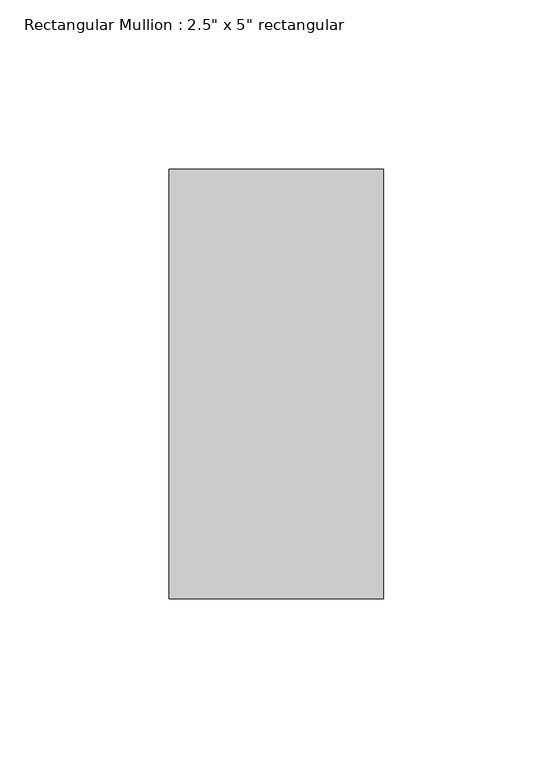
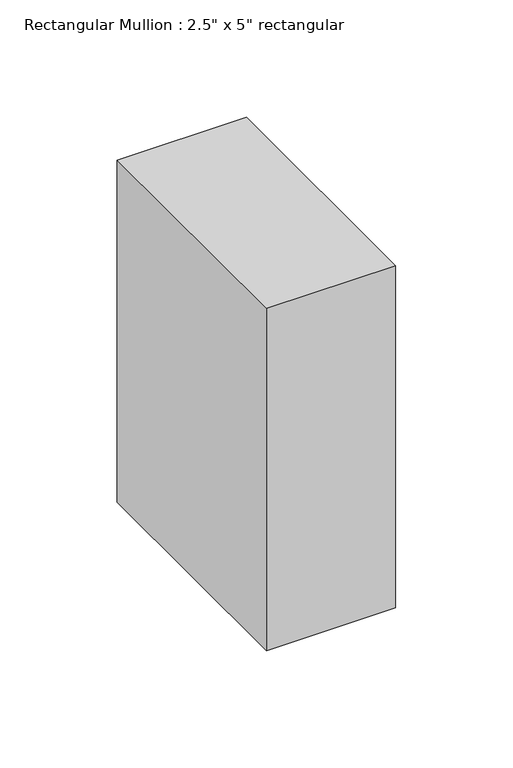
"""IFC4 building model written with IfcOpenShell, lengths in millimetres: member geometry."""

from ifc_helpers import new_model, si_unit, frame, origin, place, context, project, spatial, polyline, outline, extrude, source, transform, mapped, element, save


def member_2118ea0c(model_context):
    return source(origin(), model_context, "Body", "SweptSolid", [
        extrude(outline(polyline([(31.75, 63.5), (31.75, -63.5), (-31.75, -63.5), (-31.75, 63.5), (31.75, 63.5)])), frame((0.0, 0.0, -177.8), z_axis=(0.0, 0.0, 1.0), x_axis=(1.0, 0.0, 0.0)), (0.0, 0.0, 1.0), 177.8),
    ])


if __name__ == "__main__":
    model = new_model("IFC4")
    model_context = context("Model", 3, world=origin())
    ifc_project = project(units=[si_unit("LENGTHUNIT", "METRE", prefix="MILLI")], contexts=[model_context])
    site = spatial("IfcSite", under=ifc_project)
    building = spatial("IfcBuilding", under=site)
    placement = place(None, origin())
    member_shape = member_2118ea0c(model_context)
    element("IfcMember", 1, ObjectType="Rectangular Mullion : 2.5\" x 5\" rectangular", at=placement, inside=building, context=model_context, shape_type="MappedRepresentation", body=[
        mapped(member_shape, transform((0.0, 0.0, 0.0), x_axis=(1.0, 0.0, 0.0), y_axis=(0.0, 1.0, 0.0), z_axis=(0.0, 0.0, 1.0))),
    ])
    save(model, "model.ifc")

# Revit data of these elements
# Type "Rectangular Mullion : 2.5\" x 5\" rectangular"
#   built-in parameter 1007304 = 0.416667 (stored number, unit not read)
#   built-in parameter 1007301 = 0.104167 (stored number, unit not read)
#   built-in parameter 1007300 = 0.104167 (stored number, unit not read)
# Element 1 (IfcMember, "Rectangular Mullion : 2.5\" x 5\" rectangular")
#   Materials on its faces: "Aluminum"
# Materials
#   "Aluminum": class "Metal", colour RGB 247 247 247, transparency 0, Description = "Aluminum 6061", Cost = 0
